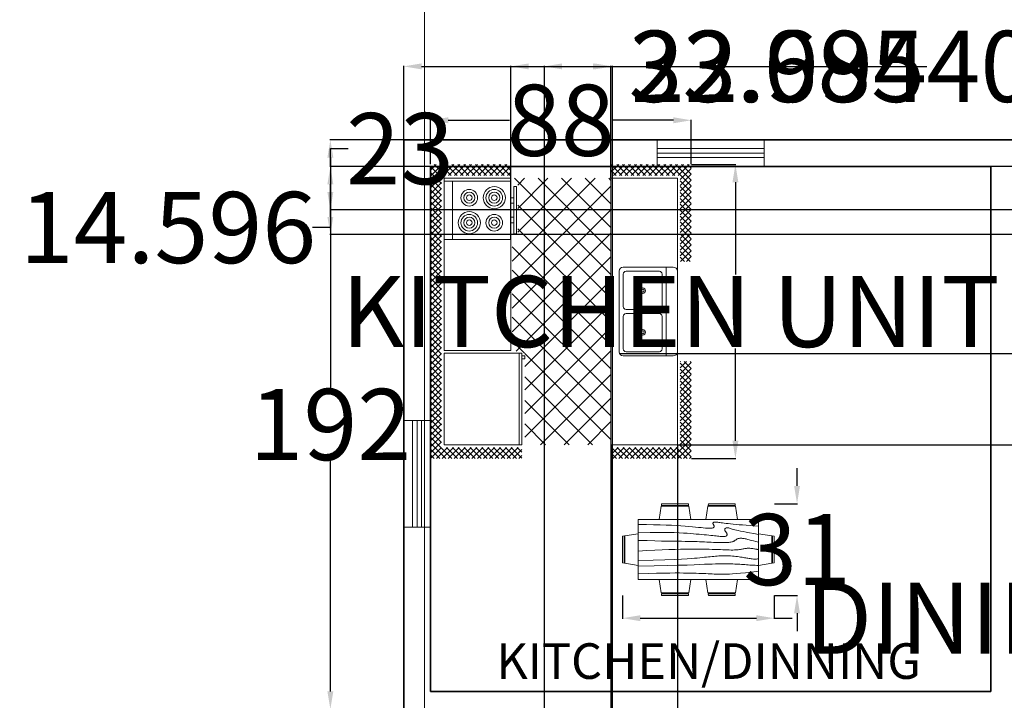
# Model space of a CAD drawing. Units: inches. Extents: x -15 to 1815, y 1023 to 2303.
# Tile 3 of 8: x 190 to 522, y 2069 to 2299. Entities that reach past the tile are written whole.
import ezdxf

# ---------------------------------------------------------------- set-up
doc = ezdxf.new("R2010")
doc.units = ezdxf.units.IN
doc.header["$MEASUREMENT"] = 0
for name, color, linetype, lineweight in [('A-ANNO-DIMS', 2, 'Continuous', 18), ('A-AREA-IDEN', 7, 'Continuous', 18), ('A-FLOR-FIXT', 9, 'Continuous', 18), ('A-FURN', 8, 'Continuous', 18), ('A-GLAZ', 4, 'Continuous', 18), ('A-REFR', 8, 'Continuous', 13), ('A-WALL', 7, 'Continuous', 35)]:
    doc.layers.add(name, color=color, linetype=linetype, lineweight=lineweight)
doc.styles.get("Standard").update_dxf_attribs({"font": 'arial.ttf'})
doc.dimstyles.get("Standard").update_dxf_attribs({"dimtxt": 24, "dimasz": 6, "dimexe": 0.18, "dimexo": 0.0625, "dimgap": 0.09, "dimtad": 0, "dimtih": 1, "dimtoh": 1, "dimdec": 0, "dimzin": 0, "dimdsep": 46, "dimlunit": 3, "dimtxsty": 'Standard', "dimcen": 0.09, "dimadec": 0, "dimazin": 0, "dimtfac": 1, "dimtdec": 0, "dimtofl": 0, "dimtmove": 0, "dimatfit": 3, "dimfxl": 1, "dimtolj": 1, "dimtzin": 0, "dimarcsym": 0})

# ---------------------------------------------------------------- blocks, each defined once
blk = doc.blocks.new('Dining Set - 36 x 72 in.')
for p, q in [((-22.2343, 26.00059), (-23.4847, 17.99762)), ((-22.2304, 26), (-5.7608, 26)), ((-22, 27.5), (-22.1562, 26.50042)), ((-5.8416, 26.5), (-22.1534, 26.5)), ((-22, 27.5), (-6, 27.5)), ((-5.8437, 26.49966), (-6, 27.5)), ((-4.5152, 17.99762), (-5.7655, 25.99926)), ((5.7657, 26.00059), (4.5153, 17.99762)), ((5.7696, 26), (22.2392, 26)), ((6, 27.5), (5.8438, 26.50042)), ((22.1584, 26.5), (5.8466, 26.5)), ((6, 27.5), (22, 27.5)), ((22.1563, 26.49966), (22, 27.5)), ((23.4848, 17.99762), (22.2345, 25.99926)), ((36, 18), (-36, 18)), ((-36, 18), (-36, -18)), ((36, -18), (36, 18)), ((-45.5, 8), (-44.5004, 8.15617)), ((-45.5, 8), (-45.5, -8)), ((-44.5, -8.15843), (-44.5, 8.15338)), ((-44.0006, 8.23428), (-35.9976, 9.48474)), ((-44, 8.23041), (-44, -8.23915)), ((44.0006, 8.23428), (35.9976, 9.48474)), ((44, 8.23041), (44, -8.23915)), ((44.5, -8.15843), (44.5, 8.15338)), ((45.5, 8), (44.5005, 8.15617)), ((45.5, 8), (45.5, -8)), ((-44.4997, -8.15631), (-45.5, -8)), ((-35.9976, -9.48476), (-43.9993, -8.2345)), ((35.9976, -9.48476), (43.9993, -8.2345)), ((44.4997, -8.15631), (45.5, -8)), ((-36, -18), (36, -18)), ((-22.2343, -26.0006), (-23.4847, -17.99762)), ((-4.5152, -17.99762), (-5.7655, -25.99928)), ((5.7657, -26.0006), (4.5153, -17.99762)), ((23.4848, -17.99762), (22.2345, -25.99928)), ((-22.2304, -26), (-5.7608, -26)), ((-22, -27.5), (-22.1562, -26.50044)), ((-5.8416, -26.5), (-22.1534, -26.5)), ((-22, -27.5), (-6, -27.5)), ((-5.8437, -26.49967), (-6, -27.5)), ((5.7696, -26), (22.2392, -26)), ((6, -27.5), (5.8438, -26.50044)), ((22.1584, -26.5), (5.8466, -26.5)), ((6, -27.5), (22, -27.5)), ((22.1563, -26.49967), (22, -27.5))]:
    blk.add_line(p, q)
for points in [[(-36, 15), (-31.1772, 14.97754), (-26.8079, 14.91406), (-22.8538, 14.81543), (-19.276, 14.6875), (-16.0362, 14.53613), (-13.0957, 14.36718), (-10.4159, 14.18652), (-7.9583, 14), (-5.6904, 13.81315), (-3.6035, 13.63021), (-1.6954, 13.45508), (0.0365, 13.29166), (1.5945, 13.14388), (2.9811, 13.01562), (4.1988, 12.9108), (5.25, 12.83333), (6.1393, 12.78613), (6.8802, 12.76823), (7.4883, 12.77767), (7.9792, 12.8125), (8.3685, 12.87077), (8.6719, 12.95052), (8.9049, 13.0498), (9.0833, 13.16666), (9.2205, 13.29899), (9.3216, 13.44401), (9.3895, 13.59879), (9.4271, 13.76041), (9.4373, 13.92594), (9.4232, 14.09245), (9.3875, 14.257), (9.3333, 14.41666), (9.2638, 14.56917), (9.1836, 14.71484), (9.0975, 14.85465), (9.0104, 14.98958), (8.9272, 15.1206), (8.8529, 15.2487), (8.7922, 15.37483), (8.75, 15.5), (8.7305, 15.62467), (8.7344, 15.74739), (8.7617, 15.86621), (8.8125, 15.97916), (8.8867, 16.08431), (8.9844, 16.17968), (9.1055, 16.26334), (9.25, 16.33333), (9.4189, 16.38802), (9.6172, 16.42708), (9.8506, 16.45052), (10.125, 16.45833), (10.4463, 16.45052), (10.8203, 16.42708), (11.2529, 16.38802), (11.75, 16.33333), (12.3184, 16.26318), (12.9694, 16.17838), (13.7151, 16.07991), (14.5677, 15.96875), (15.5395, 15.84586), (16.6426, 15.71224), (17.8893, 15.56884), (19.2917, 15.41666), (20.859, 15.25667), (22.5879, 15.08984), (24.4721, 14.91715), (26.5052, 14.73958), (28.6809, 14.5581), (30.9929, 14.3737), (33.4347, 14.18733), (36, 14)], [(-36, 10), (-28.9766, 10.14274), (-23.1725, 10.20442), (-18.4241, 10.19775), (-14.5677, 10.13541), (-11.4399, 10.03011), (-8.877, 9.89453), (-6.7154, 9.74137), (-4.7917, 9.58333), (-2.9698, 9.43082), (-1.2246, 9.28515), (0.4415, 9.14534), (2.026, 9.01041), (3.5266, 8.87939), (4.9408, 8.7513), (6.266, 8.62516), (7.5, 8.5), (8.6411, 8.37549), (9.6914, 8.2539), (10.6538, 8.13818), (11.5312, 8.03125), (12.3267, 7.93603), (13.043, 7.85547), (13.6831, 7.79248), (14.25, 7.75), (14.7471, 7.7303), (15.1797, 7.73307), (15.5537, 7.75732), (15.875, 7.80208), (16.1494, 7.86637), (16.3828, 7.94922), (16.5811, 8.04964), (16.75, 8.16666), (16.8944, 8.29915), (17.0143, 8.44531), (17.1089, 8.60319), (17.1771, 8.77083), (17.218, 8.94629), (17.2305, 9.1276), (17.2137, 9.31282), (17.1667, 9.5), (17.0895, 9.6875), (16.987, 9.875), (16.8649, 10.0625), (16.7292, 10.25), (16.5856, 10.4375), (16.4401, 10.625), (16.2985, 10.8125), (16.1667, 11), (16.05, 11.18733), (15.9518, 11.3737), (15.8752, 11.5581), (15.8229, 11.73958), (15.798, 11.91715), (15.8034, 12.08984), (15.842, 12.25667), (15.9167, 12.41666), (16.0295, 12.56836), (16.1784, 12.70833), (16.3605, 12.83268), (16.5729, 12.9375), (16.8127, 13.01888), (17.0768, 13.07291), (17.3625, 13.0957), (17.6667, 13.08333), (17.9894, 13.03312), (18.3418, 12.94726), (18.7382, 12.82918), (19.1927, 12.68229), (19.7195, 12.51001), (20.3327, 12.31575), (21.0465, 12.10294), (21.875, 11.875), (22.8357, 11.63354), (23.959, 11.37304), (25.2786, 11.08618), (26.8282, 10.76562), (28.6414, 10.40405), (30.752, 9.99414), (33.1936, 9.52856), (36, 9)], [(-36, 5.5), (-30.7157, 5.3348), (-26.069, 5.20963), (-21.9946, 5.11767), (-18.4271, 5.05208), (-15.3009, 5.00602), (-12.5508, 4.97265), (-10.1112, 4.94515), (-7.9167, 4.91666), (-5.909, 4.88167), (-4.0586, 4.83984), (-2.3429, 4.79215), (-0.7396, 4.73958), (0.7739, 4.6831), (2.22, 4.6237), (3.6213, 4.56233), (5, 4.5), (6.373, 4.43782), (7.7344, 4.3776), (9.0723, 4.32129), (10.375, 4.27083), (11.6309, 4.22819), (12.8281, 4.19531), (13.9551, 4.17415), (15, 4.16666), (15.954, 4.17448), (16.819, 4.19791), (17.6001, 4.23698), (18.3021, 4.29166), (18.9299, 4.36198), (19.4883, 4.44791), (19.9823, 4.54948), (20.4167, 4.66666), (20.7969, 4.79899), (21.1302, 4.94401), (21.4245, 5.09879), (21.6875, 5.26041), (21.9271, 5.42594), (22.1511, 5.59245), (22.3672, 5.757), (22.5834, 5.91666), (22.8065, 6.06868), (23.0404, 6.21093), (23.2879, 6.34147), (23.5521, 6.45833), (23.8358, 6.55957), (24.142, 6.64323), (24.4735, 6.70735), (24.8334, 6.75), (25.2235, 6.76969), (25.642, 6.76692), (26.0858, 6.74267), (26.5521, 6.69791), (27.0379, 6.63362), (27.5404, 6.55078), (28.0565, 6.45036), (28.5834, 6.33333), (29.1242, 6.19987), (29.7071, 6.04687), (30.3661, 5.87044), (31.1354, 5.66666), (32.0493, 5.43164), (33.142, 5.16146), (34.4475, 4.85221), (36, 4.5)], [(-36, -1), (-30.7915, -0.6591), (-26.0195, -0.38216), (-21.6519, -0.16284), (-17.6563, 0.00521), (-14.0005, 0.12833), (-10.6523, 0.21289), (-7.5796, 0.26522), (-4.75, 0.29166), (-2.134, 0.29793), (0.2878, 0.28711), (2.5317, 0.26163), (4.6146, 0.22396), (6.5529, 0.17651), (8.3633, 0.12174), (10.0623, 0.06209), (11.6667, 0), (13.1899, -0.06201), (14.6341, -0.1211), (15.9982, -0.17432), (17.2813, -0.21875), (18.4823, -0.25147), (19.6003, -0.26953), (20.6343, -0.27002), (21.5834, -0.25), (22.4481, -0.20768), (23.2357, -0.14584), (23.9549, -0.06836), (24.6146, 0.02083), (25.2235, 0.11784), (25.7904, 0.21875), (26.3241, 0.31966), (26.8334, 0.41666), (27.3265, 0.50618), (27.8099, 0.58593), (28.2894, 0.65397), (28.7709, 0.70833), (29.2601, 0.74707), (29.763, 0.76823), (30.2855, 0.76985), (30.8334, 0.75), (31.4088, 0.70784), (31.9994, 0.64713), (32.589, 0.57275), (33.1615, 0.48958), (33.7008, 0.4025), (34.1908, 0.3164), (34.6153, 0.23616), (34.9584, 0.16666), (35.2099, 0.11165), (35.3848, 0.07031), (35.504, 0.04069), (35.5886, 0.02083), (35.6594, 0.00879), (35.7377, 0.0026), (35.8442, 0.00032), (36, 0)], [(-36, -6.5), (-27.1843, -6.31267), (-20.084, -6.1263), (-14.469, -5.9419), (-10.1094, -5.76042), (-6.7752, -5.58285), (-4.2363, -5.41016), (-2.2629, -5.24333), (-0.625, -5.08334), (0.8708, -4.93099), (2.2715, -4.78646), (3.5872, -4.64974), (4.8281, -4.52084), (6.0046, -4.39974), (7.127, -4.28646), (8.2053, -4.18099), (9.25, -4.08334), (10.2705, -3.99382), (11.2734, -3.91407), (12.2647, -3.84603), (13.25, -3.79167), (14.2354, -3.75293), (15.2266, -3.73177), (16.2295, -3.73015), (17.25, -3.75), (18.2912, -3.79248), (19.3451, -3.85547), (20.4009, -3.93604), (21.4479, -4.03125), (22.4754, -4.13819), (23.4727, -4.25391), (24.4289, -4.37549), (25.3334, -4.5), (26.1785, -4.62492), (26.9694, -4.74935), (27.7145, -4.87281), (28.4219, -4.99479), (29.1, -5.11483), (29.7572, -5.23242), (30.4016, -5.34709), (31.0417, -5.45834), (31.6837, -5.56437), (32.3262, -5.65821), (32.9658, -5.73153), (33.599, -5.77604), (34.2224, -5.78345), (34.8327, -5.74545), (35.4264, -5.65373), (36, -5.5)], [(-36, -10), (-26.4022, -9.81299), (-18.4675, -9.62891), (-11.9839, -9.45069), (-6.7396, -9.28125), (-2.5226, -9.12354), (0.8789, -8.98047), (3.6769, -8.85498), (6.0833, -8.75), (8.2767, -8.66765), (10.3021, -8.60677), (12.1712, -8.56543), (13.8958, -8.54167), (15.4876, -8.53353), (16.9583, -8.53907), (18.3197, -8.55632), (19.5834, -8.58334), (20.7616, -8.61841), (21.8685, -8.66081), (22.9188, -8.71004), (23.9271, -8.76563), (24.9081, -8.82707), (25.8763, -8.89388), (26.8465, -8.96558), (27.8334, -9.04167), (28.8474, -9.12118), (29.8828, -9.20117), (30.93, -9.27824), (31.9792, -9.34896), (33.0205, -9.40991), (34.0443, -9.45768), (35.0407, -9.48885), (36, -9.5)], [(-36, -14.5), (-30.0881, -14.33513), (-25.0332, -14.21224), (-20.7312, -14.12647), (-17.0781, -14.07292), (-13.97, -14.04671), (-11.3027, -14.04297), (-8.9724, -14.05681), (-6.875, -14.08334), (-4.9224, -14.11833), (-3.0905, -14.16016), (-1.3709, -14.20785), (0.2448, -14.26042), (1.7647, -14.3169), (3.1973, -14.3763), (4.5507, -14.43767), (5.8333, -14.5), (7.0554, -14.5621), (8.235, -14.62175), (9.3922, -14.67652), (10.5469, -14.72396), (11.7192, -14.76164), (12.929, -14.78711), (14.1965, -14.79794), (15.5417, -14.79167), (16.9933, -14.76424), (18.6152, -14.70508), (20.4804, -14.60197), (22.6615, -14.44271), (25.2312, -14.21509), (28.2624, -13.9069), (31.8277, -13.50594), (36, -13)]]:
    blk.add_lwpolyline(points)
blk = doc.blocks.new('Kitchen Layout - 7 x 8 ft')
for p, q in [((-5, 81.32), (2.68, 89)), ((-5, 83.44), (0.56, 89)), ((-5, 85.56), (-1.56, 89)), ((-5, 87.68), (-3.68, 89)), ((-1, 84.97), (-5, 88.97)), ((1.09, 85), (-2.91, 89)), ((3.21, 85), (-0.79, 89)), ((0.81, 85), (4.81, 89)), ((5.34, 85), (1.34, 89)), ((2.93, 85), (6.93, 89)), ((7.46, 85), (3.46, 89)), ((5.05, 85), (9.05, 89)), ((9.58, 85), (5.58, 89)), ((7.17, 85), (11.17, 89)), ((11.7, 85), (7.7, 89)), ((9.29, 85), (13.29, 89)), ((13.82, 85), (9.82, 89)), ((11.41, 85), (15.41, 89)), ((15.94, 85), (11.94, 89)), ((13.53, 85), (17.53, 89)), ((18.06, 85), (14.06, 89)), ((15.65, 85), (19.65, 89)), ((20.18, 85), (16.18, 89)), ((17.78, 85), (21.78, 89)), ((22.31, 85), (18.31, 89)), ((19.9, 85), (23.9, 89)), ((24.43, 85), (20.43, 89)), ((22.02, 85), (26.02, 89)), ((26.55, 85), (22.55, 89)), ((24.14, 85), (28.14, 89)), ((28.67, 85), (24.67, 89)), ((26.26, 85), (30.26, 89)), ((30.79, 85), (26.79, 89)), ((28.38, 85), (32.38, 89)), ((32.91, 85), (28.91, 89)), ((30.5, 85), (34.5, 89)), ((35.03, 85), (31.03, 89)), ((32.63, 85), (36.63, 89)), ((37.16, 85), (33.16, 89)), ((34.75, 85), (38.75, 89)), ((39.28, 85), (35.28, 89)), ((36.87, 85), (40.87, 89)), ((41.4, 85), (37.4, 89)), ((38.99, 85), (42.99, 89)), ((43.52, 85), (39.52, 89)), ((41.11, 85), (45.11, 89)), ((45.64, 85), (41.64, 89)), ((43.23, 85), (47.23, 89)), ((47.76, 85), (43.76, 89)), ((45.35, 85), (49.35, 89)), ((49.88, 85), (45.88, 89)), ((47.47, 85), (51.47, 89)), ((52, 85), (48, 89)), ((49.6, 85), (53.6, 89)), ((54.13, 85), (50.13, 89)), ((51.72, 85), (55.72, 89)), ((56.25, 85), (52.25, 89)), ((53.84, 85), (57.84, 89)), ((58.37, 85), (54.37, 89)), ((55.96, 85), (59.96, 89)), ((60.49, 85), (56.49, 89)), ((58.08, 85), (62.08, 89)), ((62.61, 85), (58.61, 89)), ((60.2, 85), (64.2, 89)), ((64.73, 85), (60.73, 89)), ((62.32, 85), (66.32, 89)), ((66.85, 85), (62.85, 89)), ((64.45, 85), (68.45, 89)), ((68.97, 85), (64.97, 89)), ((66.57, 85), (70.57, 89)), ((71.1, 85), (67.1, 89)), ((68.69, 85), (72.69, 89)), ((73.22, 85), (69.22, 89)), ((70.81, 85), (74.81, 89)), ((75.34, 85), (71.34, 89)), ((72.93, 85), (76.93, 89)), ((77.46, 85), (73.46, 89)), ((75.05, 85), (79.05, 89)), ((79.58, 85), (75.58, 89)), ((77.17, 85), (81.17, 89)), ((81.7, 85), (77.7, 89)), ((79.29, 85), (83.29, 89)), ((83.82, 85), (79.82, 89)), ((81.42, 85), (85.42, 89)), ((85.95, 85), (81.95, 89)), ((83.54, 85), (87.54, 89)), ((88.07, 85), (84.07, 89)), ((85.66, 85), (89.66, 89)), ((90.19, 85), (86.19, 89)), ((87.78, 85), (91.78, 89)), ((92.31, 85), (88.31, 89)), ((89.9, 85), (93.9, 89)), ((94.43, 85), (90.43, 89)), ((92.02, 85), (96.02, 89)), ((96.55, 85), (92.55, 89)), ((94.14, 85), (98.14, 89)), ((101, 82.67), (94.67, 89)), ((96.27, 85), (100.27, 89)), ((101, 84.79), (96.79, 89)), ((101, 86.92), (98.92, 89)), ((-1, 82.85), (-5, 86.85)), ((97, 83.61), (101, 87.61)), ((97, 81.49), (101, 85.49)), ((-1, 80.73), (-5, 84.73)), ((-5, 79.19), (-1, 83.19)), ((-1, 78.61), (-5, 82.61)), ((34, 84), (96, 84)), ((34, 60), (34, 84)), ((96, 84), (96, 60)), ((101, 80.55), (97, 84.55)), ((97, 79.37), (101, 83.37)), ((101, 78.43), (97, 82.43)), ((-5, 77.07), (-1, 81.07)), ((-1, 76.49), (-5, 80.49)), ((-5, 74.95), (-1, 78.95)), ((-1, 74.36), (-5, 78.36)), ((74, 81), (95, 81)), ((97, 77.25), (101, 81.25)), ((101, 76.31), (97, 80.31)), ((97, 75.13), (101, 79.13)), ((101, 74.19), (97, 78.19)), ((-5, 72.83), (-1, 76.83)), ((-1, 72.24), (-5, 76.24)), ((-5, 70.71), (-1, 74.71)), ((97, 73.01), (101, 77.01)), ((101, 72.07), (97, 76.07)), ((97, 70.89), (101, 74.89)), ((-1, 70.12), (-5, 74.12)), ((-5, 68.59), (-1, 72.59)), ((-1, 68), (-5, 72)), ((101, 69.95), (97, 73.95)), ((97, 68.76), (101, 72.76)), ((101, 67.82), (97, 71.82)), ((-5, 66.47), (-1, 70.47)), ((-1, 65.88), (-5, 69.88)), ((-5, 64.35), (-1, 68.35)), ((-1, 63.76), (-5, 67.76)), ((97, 66.64), (101, 70.64)), ((101, 65.7), (97, 69.7)), ((97, 64.52), (101, 68.52)), ((101, 63.58), (97, 67.58)), ((-5, 62.22), (-1, 66.22)), ((-1, 61.64), (-5, 65.64)), ((-5, 60.1), (-1, 64.1)), ((97, 62.4), (101, 66.4)), ((101, 61.46), (97, 65.46)), ((97, 60.28), (101, 64.28)), ((-1, 59.52), (-5, 63.52)), ((-5, 57.98), (-1, 61.98)), ((-1, 57.39), (-5, 61.39)), ((100.34, 60), (97, 63.34)), ((98.22, 60), (97, 61.22)), ((98.84, 60), (101, 62.16)), ((-1.73, 56), (-5, 59.27)), ((-3.85, 56), (-5, 57.15)), ((-4.86, 56), (-1, 59.86)), ((-2.74, 56), (-1, 57.74)), ((0, 57), (33, 57)), ((10.4, 24), (45.9, 59.5)), ((18.88, 24), (54.38, 59.5)), ((27.37, 24), (62.87, 59.5)), ((33.03, 55.11), (37.41, 59.5)), ((67.71, 24), (33.68, 58.04)), ((96, 60), (34, 60)), ((35.85, 24), (71.35, 59.5)), ((76.2, 24), (40.7, 59.5)), ((44.34, 24), (77.84, 57.5)), ((84.68, 24), (49.18, 59.5)), ((52.82, 24), (86.32, 57.5)), ((93.17, 24), (57.67, 59.5)), ((61.31, 24), (96, 58.69)), ((96, 29.65), (66.15, 59.5)), ((96, 38.14), (76.64, 57.5)), ((80, 60), (80, 59)), ((82, 59), (82, 60)), ((96, 46.63), (85.13, 57.5)), ((87, 59), (87, 60)), ((89, 60), (89, 59)), ((96, 55.11), (93.57, 57.54)), ((100.96, 60), (101, 60.04)), ((0, 30.57), (24.43, 55)), ((0, 39.06), (15.94, 55)), ((0, 47.54), (7.46, 55)), ((1.91, 24), (32.91, 55)), ((33.77, 24), (2.77, 55)), ((42.26, 24), (11.26, 55)), ((50.74, 24), (19.74, 55)), ((59.23, 24), (28.23, 55)), ((31, 55), (31, 56)), ((32, 55), (31, 55)), ((32, 56), (32, 55)), ((69.79, 24), (96, 50.21)), ((25.29, 24), (0, 49.29)), ((16.8, 24), (0, 40.8)), ((78.28, 24), (96, 41.72)), ((8.32, 24), (0, 32.32)), ((86.76, 24), (96, 33.24)), ((-5, 21.92), (-2.92, 24)), ((-5, 19.8), (-1, 23.8)), ((-1, 19.21), (-5, 23.21)), ((-5, 17.68), (-1, 21.68)), ((-1, 21.33), (-3.67, 24)), ((-1, 23.45), (-1.55, 24)), ((0, 24), (96, 24)), ((0, 0), (0, 24)), ((95.25, 24), (96, 24.75)), ((96, 24), (96, 0)), ((97, 22.1), (98.9, 24)), ((97, 19.97), (101, 23.97)), ((101, 19.03), (97, 23.03)), ((97, 17.85), (101, 21.85)), ((101, 21.16), (98.16, 24)), ((101, 23.28), (100.28, 24)), ((-1, 17.09), (-5, 21.09)), ((-5, 15.55), (-1, 19.55)), ((-1, 14.97), (-5, 18.97)), ((47.25, 6.5), (47.25, 18.5)), ((48.75, 18.5), (48.75, 6.5)), ((101, 16.91), (97, 20.91)), ((97, 15.73), (101, 19.73)), ((101, 14.79), (97, 18.79)), ((-5, 13.43), (-1, 17.43)), ((-1, 12.85), (-5, 16.85)), ((-5, 11.31), (-1, 15.31)), ((-1, 10.73), (-5, 14.73)), ((97, 13.61), (101, 17.61)), ((101, 12.67), (97, 16.67)), ((97, 11.49), (101, 15.49)), ((101, 10.55), (97, 14.55)), ((-5, 9.19), (-1, 13.19)), ((-1, 8.6), (-5, 12.6)), ((-5, 7.07), (-1, 11.07)), ((97, 9.37), (101, 13.37)), ((101, 8.43), (97, 12.43)), ((97, 7.25), (101, 11.25)), ((-1, 6.48), (-5, 10.48)), ((-5, 4.95), (-1, 8.95)), ((-1, 4.36), (-5, 8.36)), ((101, 6.31), (97, 10.31)), ((97, 5.12), (101, 9.12)), ((101, 4.18), (97, 8.18)), ((-5, 2.83), (-1, 6.83)), ((-1, 2.24), (-5, 6.24)), ((-5, 0.71), (-1, 4.71)), ((-1, 0.12), (-5, 4.12)), ((64, 4), (32, 4)), ((97, 3), (101, 7)), ((101, 2.06), (97, 6.06)), ((97, 0.88), (101, 4.88)), ((101, -0.06), (97, 3.94)), ((-5, -1.42), (-1, 2.58)), ((2, -5), (-5, 2)), ((-5, -3.54), (-1, 0.46)), ((96, 0), (0, 0)), ((93.24, -5), (101, 2.76)), ((95.36, -5), (101, 0.64)), ((101, -2.18), (97, 1.82)), ((-0.12, -5), (-5, -0.12)), ((-2.25, -5), (-5, -2.25)), ((-4.34, -5), (-0.34, -1)), ((-2.22, -5), (1.78, -1)), ((-0.1, -5), (3.9, -1)), ((4.12, -5), (0.12, -1)), ((2.02, -5), (6.02, -1)), ((6.24, -5), (2.24, -1)), ((4.14, -5), (8.14, -1)), ((8.36, -5), (4.36, -1)), ((6.27, -5), (10.27, -1)), ((10.48, -5), (6.48, -1)), ((8.39, -5), (12.39, -1)), ((12.6, -5), (8.6, -1)), ((10.51, -5), (14.51, -1)), ((14.73, -5), (10.73, -1)), ((12.63, -5), (16.63, -1)), ((16.85, -5), (12.85, -1)), ((14.75, -5), (18.75, -1)), ((18.97, -5), (14.97, -1)), ((16.87, -5), (20.87, -1)), ((21.09, -5), (17.09, -1)), ((18.99, -5), (22.99, -1)), ((23.21, -5), (19.21, -1)), ((21.11, -5), (25.11, -1)), ((25.33, -5), (21.33, -1)), ((23.24, -5), (27.24, -1)), ((27.45, -5), (23.45, -1)), ((25.36, -5), (29.36, -1)), ((29.57, -5), (25.57, -1)), ((27.48, -5), (30, -2.48)), ((30, -3.3), (27.7, -1)), ((30, -1.18), (29.82, -1)), ((66, -2.54), (67.54, -1)), ((66, -4.66), (69.66, -1)), ((69.88, -5), (66, -1.12)), ((67.76, -5), (66, -3.24)), ((67.78, -5), (71.78, -1)), ((72, -5), (68, -1)), ((69.9, -5), (73.9, -1)), ((74.12, -5), (70.12, -1)), ((72.03, -5), (76.03, -1)), ((76.24, -5), (72.24, -1)), ((74.15, -5), (78.15, -1)), ((78.36, -5), (74.36, -1)), ((76.27, -5), (80.27, -1)), ((80.49, -5), (76.49, -1)), ((78.39, -5), (82.39, -1)), ((82.61, -5), (78.61, -1)), ((80.51, -5), (84.51, -1)), ((84.73, -5), (80.73, -1)), ((82.63, -5), (86.63, -1)), ((86.85, -5), (82.85, -1)), ((84.75, -5), (88.75, -1)), ((88.97, -5), (84.97, -1)), ((86.88, -5), (90.88, -1)), ((91.09, -5), (87.09, -1)), ((89, -5), (93, -1)), ((93.21, -5), (89.21, -1)), ((91.12, -5), (95.12, -1)), ((95.34, -5), (91.34, -1)), ((97.46, -5), (93.46, -1)), ((99.58, -5), (95.58, -1)), ((101, -4.3), (97, -0.3)), ((97.48, -5), (101, -1.48)), ((-4.37, -5), (-5, -4.37)), ((29.6, -5), (30, -4.6)), ((99.6, -5), (101, -3.6))]:
    blk.add_line(p, q)
for points in [[(0, 56), (0, 84), (33, 84), (33, 56)], [(74, 60), (74, 84), (95, 84), (95, 60)], [(76, 58), (76, 59), (93, 59), (93, 58)]]:
    blk.add_lwpolyline(points, close=True)
for points in [[(32, 1.5), (32, 19.5)], [(33.5, 21), (62.5, 21)], [(33.5, 6.5), (33.5, 18.5)], [(34.5, 19.5), (46.25, 19.5)], [(49.75, 19.5), (61.5, 19.5)], [(62.5, 18.5), (62.5, 6.5)], [(64, 19.5), (64, 1.5)], [(46.25, 5.5), (34.5, 5.5)], [(61.5, 5.5), (49.75, 5.5)], [(62.5, 0), (33.5, 0)]]:
    blk.add_lwpolyline(points)
for centre, radius in [((80, 75), 4), ((80, 75), 3), ((80, 75), 2), ((80, 75), 1), ((89, 75), 3), ((89, 75), 2), ((89, 75), 1), ((80, 66), 3), ((80, 66), 2), ((89, 66), 4), ((89, 66), 3), ((89, 66), 2), ((80, 66), 1), ((89, 66), 1), ((40.5, 12.5), 1), ((40.5, 12.5), 0.5), ((55.5, 12.5), 1), ((55.5, 12.5), 0.5)]:
    blk.add_circle(centre, radius)
for centre, radius, start, end in [((33.5, 19.5), 1.5, 90, 180), ((34.5, 18.5), 1, 90, 180), ((46.25, 18.5), 1, 0, 90), ((49.75, 18.5), 1, 90, 180), ((61.5, 18.5), 1, 0, 90), ((62.5, 19.5), 1.5, 0, 90), ((34.5, 6.5), 1, 180, 270), ((46.25, 6.5), 1, 270, 0), ((49.75, 6.5), 1, 180, 270), ((61.5, 6.5), 1, 270, 0), ((33.5, 1.5), 1.5, 180, 270), ((62.5, 1.5), 1.5, 270, 0)]:
    blk.add_arc(centre, radius, start, end)
blk = doc.blocks.new('Window - Wood Frame 36 in. Wide plan')
for p, q in [((0, 7.5), (0, -1.5)), ((36, 7.5), (36, -1.5)), ((0, 4.5), (36, 4.5)), ((0, 3), (36, 3)), ((0, 1.5), (36, 1.5))]:
    blk.add_line(p, q)
blk = doc.blocks.new('*D33')
at = {"layer": 'A-ANNO-DIMS', "color": 0, "lineweight": -2, "transparency": 16777216}
for p, q in [((393.59, 2104.63), (393.59, 2096.83)), ((444.77, 2104.63), (444.77, 2096.83)), ((399.59, 2097.01), (438.77, 2097.01)), ((444.77, 2097.01), (450.77, 2097.01))]:
    blk.add_line(p, q, dxfattribs=at)
at = {"layer": 'A-ANNO-DIMS', "color": 0, "transparency": 16777216}
for points in [[(399.59, 2098.01), (399.59, 2096.01), (393.59, 2097.01)], [(438.77, 2098.01), (438.77, 2096.01), (444.77, 2097.01)]]:
    blk.add_solid(points, dxfattribs=at)
at = {"layer": 'Defpoints', "color": 0, "transparency": 16777216}
for p in [(393.59, 2104.69), (444.77, 2104.69), (444.77, 2097.01)]:
    blk.add_point(p, dxfattribs=at)
at = {"layer": 'A-ANNO-DIMS', "color": 0, "transparency": 16777216, "insert": (565.73, 2097.01), "char_height": 24, "attachment_point": 5}
blk.add_mtext('\\A1;DINING SET 51', dxfattribs=at)
blk = doc.blocks.new('*D34')
at = {"layer": 'A-ANNO-DIMS', "color": 0, "lineweight": -2, "transparency": 16777216}
for p, q in [((452.45, 2141.62), (452.45, 2147.62)), ((444.83, 2135.62), (452.63, 2135.62)), ((444.83, 2104.69), (452.63, 2104.69)), ((452.45, 2098.69), (452.45, 2092.69))]:
    blk.add_line(p, q, dxfattribs=at)
at = {"layer": 'A-ANNO-DIMS', "color": 0, "transparency": 16777216}
for points in [[(451.45, 2141.62), (453.45, 2141.62), (452.45, 2135.62)], [(451.45, 2098.69), (453.45, 2098.69), (452.45, 2104.69)]]:
    blk.add_solid(points, dxfattribs=at)
at = {"layer": 'Defpoints', "color": 0, "transparency": 16777216}
for p in [(444.77, 2135.62), (452.45, 2135.62), (444.77, 2104.69)]:
    blk.add_point(p, dxfattribs=at)
at = {"layer": 'A-ANNO-DIMS', "color": 0, "transparency": 16777216, "insert": (452.45, 2120.16), "char_height": 24, "attachment_point": 5}
blk.add_mtext('\\A1;31', dxfattribs=at)
blk = doc.blocks.new('*D39')
at = {"layer": 'A-ANNO-DIMS', "color": 0, "lineweight": -2, "transparency": 16777216}
for p, q in [((416.85, 2250.01), (431.85, 2250.01)), ((431.67, 2244.01), (431.67, 2212.92)), ((431.67, 2156.83), (431.67, 2187.92)), ((416.85, 2150.83), (431.85, 2150.83))]:
    blk.add_line(p, q, dxfattribs=at)
at = {"layer": 'A-ANNO-DIMS', "color": 0, "transparency": 16777216}
for points in [[(430.67, 2244.01), (432.67, 2244.01), (431.67, 2250.01)], [(430.67, 2156.83), (432.67, 2156.83), (431.67, 2150.83)]]:
    blk.add_solid(points, dxfattribs=at)
at = {"layer": 'Defpoints', "color": 0, "transparency": 16777216}
for p in [(416.79, 2250.01), (431.67, 2250.01), (416.79, 2150.83)]:
    blk.add_point(p, dxfattribs=at)
at = {"layer": 'A-ANNO-DIMS', "color": 0, "transparency": 16777216, "insert": (431.67, 2200.42), "char_height": 24, "attachment_point": 5}
blk.add_mtext('\\A1;KITCHEN UNIT 99', dxfattribs=at)
blk = doc.blocks.new('*D40')
at = {"layer": 'A-ANNO-DIMS', "color": 0, "lineweight": -2, "transparency": 16777216}
for p, q in [((328.83, 2250.08), (328.83, 2265.07)), ((334.83, 2264.89), (355.49, 2264.89)), ((410.79, 2264.89), (390.13, 2264.89)), ((416.79, 2250.08), (416.79, 2265.07))]:
    blk.add_line(p, q, dxfattribs=at)
at = {"layer": 'A-ANNO-DIMS', "color": 0, "transparency": 16777216}
for points in [[(334.83, 2265.89), (334.83, 2263.89), (328.83, 2264.89)], [(410.79, 2265.89), (410.79, 2263.89), (416.79, 2264.89)]]:
    blk.add_solid(points, dxfattribs=at)
at = {"layer": 'Defpoints', "color": 0, "transparency": 16777216}
for p in [(328.83, 2264.89), (328.83, 2250.01), (416.79, 2250.01)]:
    blk.add_point(p, dxfattribs=at)
at = {"layer": 'A-ANNO-DIMS', "color": 0, "transparency": 16777216, "insert": (372.81, 2264.89), "char_height": 24, "attachment_point": 5}
blk.add_mtext('\\A1;88', dxfattribs=at)
blk = doc.blocks.new('*D59')
at = {"layer": 'A-ANNO-DIMS', "color": 0, "lineweight": -2, "transparency": 16777216}
for p, q in [((319.83, 2258.39), (319.83, 2283.24)), ((325.83, 2283.06), (496.25, 2283.06)), ((720.83, 2283.06), (550.42, 2283.06)), ((726.83, 2258.39), (726.83, 2283.24))]:
    blk.add_line(p, q, dxfattribs=at)
at = {"layer": 'A-ANNO-DIMS', "color": 0, "transparency": 16777216}
for points in [[(325.83, 2284.06), (325.83, 2282.06), (319.83, 2283.06)], [(720.83, 2284.06), (720.83, 2282.06), (726.83, 2283.06)]]:
    blk.add_solid(points, dxfattribs=at)
at = {"layer": 'Defpoints', "color": 0, "transparency": 16777216}
for p in [(726.83, 2283.06), (319.83, 2258.33), (726.83, 2258.33)]:
    blk.add_point(p, dxfattribs=at)
at = {"layer": 'A-ANNO-DIMS', "color": 0, "transparency": 16777216, "insert": (523.33, 2283.06), "char_height": 24, "attachment_point": 5}
blk.add_mtext('\\A1;407', dxfattribs=at)
blk = doc.blocks.new('*D63')
at = {"layer": 'A-ANNO-DIMS', "color": 0, "lineweight": -2, "transparency": 16777216}
for p, q in [((319.77, 2258.33), (294.92, 2258.33)), ((295.1, 2252.33), (295.1, 2174.67)), ((295.1, 2072.33), (295.1, 2149.98)), ((319.77, 2066.33), (294.92, 2066.33))]:
    blk.add_line(p, q, dxfattribs=at)
at = {"layer": 'A-ANNO-DIMS', "color": 0, "transparency": 16777216}
for points in [[(294.1, 2252.33), (296.1, 2252.33), (295.1, 2258.33)], [(294.1, 2072.33), (296.1, 2072.33), (295.1, 2066.33)]]:
    blk.add_solid(points, dxfattribs=at)
at = {"layer": 'Defpoints', "color": 0, "transparency": 16777216}
for p in [(295.1, 2258.33), (319.83, 2258.33), (319.83, 2066.33)]:
    blk.add_point(p, dxfattribs=at)
at = {"layer": 'A-ANNO-DIMS', "color": 0, "transparency": 16777216, "insert": (295.1, 2162.33), "char_height": 24, "attachment_point": 5}
blk.add_mtext('\\A1;192', dxfattribs=at)
blk = doc.blocks.new('*D68')
at = {"layer": 'A-ANNO-DIMS', "color": 0, "lineweight": -2, "transparency": 16777216}
for p, q in [((367.25, 1964.98), (367.25, 2283.24)), ((373.25, 2283.06), (384.24, 2283.06)), ((390.24, 1945.2), (390.24, 2283.24)), ((390.24, 2283.06), (396.24, 2283.06))]:
    blk.add_line(p, q, dxfattribs=at)
at = {"layer": 'A-ANNO-DIMS', "color": 0, "transparency": 16777216}
for points in [[(373.25, 2284.06), (373.25, 2282.06), (367.25, 2283.06)], [(384.24, 2284.06), (384.24, 2282.06), (390.24, 2283.06)]]:
    blk.add_solid(points, dxfattribs=at)
at = {"layer": 'Defpoints', "color": 0, "transparency": 16777216}
for p in [(390.24, 2283.06), (367.25, 1964.92), (390.24, 1945.14)]:
    blk.add_point(p, dxfattribs=at)
at = {"layer": 'A-ANNO-DIMS', "color": 0, "transparency": 16777216, "insert": (446.3, 2283.06), "char_height": 24, "attachment_point": 5}
blk.add_mtext('\\A1;22.994', dxfattribs=at)
blk = doc.blocks.new('*D74')
at = {"layer": 'A-ANNO-DIMS', "color": 0, "lineweight": -2, "transparency": 16777216}
for p, q in [((295.1, 2249.33), (295.1, 2255.33)), ((295.1, 2255.33), (301.1, 2255.33)), ((623.77, 2249.33), (294.92, 2249.33)), ((295.1, 2232.33), (295.1, 2243.33)), ((681.77, 2226.33), (294.92, 2226.33))]:
    blk.add_line(p, q, dxfattribs=at)
at = {"layer": 'A-ANNO-DIMS', "color": 0, "transparency": 16777216}
for points in [[(294.1, 2243.33), (296.1, 2243.33), (295.1, 2249.33)], [(294.1, 2232.33), (296.1, 2232.33), (295.1, 2226.33)]]:
    blk.add_solid(points, dxfattribs=at)
at = {"layer": 'Defpoints', "color": 0, "transparency": 16777216}
for p in [(295.1, 2249.33), (623.83, 2249.33), (681.83, 2226.33)]:
    blk.add_point(p, dxfattribs=at)
at = {"layer": 'A-ANNO-DIMS', "color": 0, "transparency": 16777216, "insert": (318.59, 2255.33), "char_height": 24, "attachment_point": 5}
blk.add_mtext('\\A1;23', dxfattribs=at)
blk = doc.blocks.new('*D76')
at = {"layer": 'A-ANNO-DIMS', "color": 0, "lineweight": -2, "transparency": 16777216}
for p, q in [((523.77, 2249.33), (294.92, 2249.33)), ((295.1, 2243.33), (295.1, 2240.73)), ((543.56, 2234.73), (294.92, 2234.73)), ((295.1, 2234.73), (295.1, 2228.73)), ((295.1, 2228.73), (289.1, 2228.73))]:
    blk.add_line(p, q, dxfattribs=at)
at = {"layer": 'A-ANNO-DIMS', "color": 0, "transparency": 16777216}
for points in [[(294.1, 2243.33), (296.1, 2243.33), (295.1, 2249.33)], [(294.1, 2240.73), (296.1, 2240.73), (295.1, 2234.73)]]:
    blk.add_solid(points, dxfattribs=at)
at = {"layer": 'Defpoints', "color": 0, "transparency": 16777216}
for p in [(523.83, 2249.33), (295.1, 2234.73), (543.62, 2234.73)]:
    blk.add_point(p, dxfattribs=at)
at = {"layer": 'A-ANNO-DIMS', "color": 0, "transparency": 16777216, "insert": (240.33, 2228.73), "char_height": 24, "attachment_point": 5}
blk.add_mtext('\\A1;14.596', dxfattribs=at)
blk = doc.blocks.new('*D77')
at = {"layer": 'A-ANNO-DIMS', "color": 0, "lineweight": -2, "transparency": 16777216}
for p, q in [((355.97, 2224.81), (355.97, 2283.24)), ((361.97, 2283.06), (383.65, 2283.06)), ((389.65, 2245.4), (389.65, 2283.24)), ((389.65, 2283.06), (395.65, 2283.06))]:
    blk.add_line(p, q, dxfattribs=at)
at = {"layer": 'A-ANNO-DIMS', "color": 0, "transparency": 16777216}
for points in [[(361.97, 2284.06), (361.97, 2282.06), (355.97, 2283.06)], [(383.65, 2284.06), (383.65, 2282.06), (389.65, 2283.06)]]:
    blk.add_solid(points, dxfattribs=at)
at = {"layer": 'Defpoints', "color": 0, "transparency": 16777216}
for p in [(389.65, 2283.06), (389.65, 2245.34), (355.97, 2224.75)]:
    blk.add_point(p, dxfattribs=at)
at = {"layer": 'A-ANNO-DIMS', "color": 0, "transparency": 16777216, "insert": (445.64, 2283.06), "char_height": 24, "attachment_point": 5}
blk.add_mtext('\\A1;33.685', dxfattribs=at)
blk = doc.blocks.new('*D78')
at = {"layer": 'A-ANNO-DIMS', "color": 0, "lineweight": -2, "transparency": 16777216}
for p, q in [((389.65, 2155.45), (389.65, 1800.41)), ((412.11, 2155.45), (412.11, 1800.41)), ((395.65, 1800.59), (406.11, 1800.59)), ((412.11, 1800.59), (418.11, 1800.59))]:
    blk.add_line(p, q, dxfattribs=at)
at = {"layer": 'A-ANNO-DIMS', "color": 0, "transparency": 16777216}
for points in [[(395.65, 1801.59), (395.65, 1799.59), (389.65, 1800.59)], [(406.11, 1801.59), (406.11, 1799.59), (412.11, 1800.59)]]:
    blk.add_solid(points, dxfattribs=at)
at = {"layer": 'Defpoints', "color": 0, "transparency": 16777216}
for p in [(389.65, 2155.51), (412.11, 2155.51), (412.11, 1800.59)]:
    blk.add_point(p, dxfattribs=at)
at = {"layer": 'A-ANNO-DIMS', "color": 0, "transparency": 16777216, "insert": (468.22, 1800.59), "char_height": 24, "attachment_point": 5}
blk.add_mtext('\\A1;22.457', dxfattribs=at)
blk = doc.blocks.new('*D79')
at = {"layer": 'A-ANNO-DIMS', "color": 0, "lineweight": -2, "transparency": 16777216}
for p, q in [((751.57, 2192.31), (751.57, 2198.31)), ((392.63, 2186.31), (751.75, 2186.31)), ((412.17, 2155.51), (751.75, 2155.51)), ((751.57, 2149.51), (751.57, 2143.51))]:
    blk.add_line(p, q, dxfattribs=at)
at = {"layer": 'A-ANNO-DIMS', "color": 0, "transparency": 16777216}
for points in [[(750.57, 2192.31), (752.57, 2192.31), (751.57, 2186.31)], [(750.57, 2149.51), (752.57, 2149.51), (751.57, 2155.51)]]:
    blk.add_solid(points, dxfattribs=at)
at = {"layer": 'Defpoints', "color": 0, "transparency": 16777216}
for p in [(392.57, 2186.31), (412.11, 2155.51), (751.57, 2155.51)]:
    blk.add_point(p, dxfattribs=at)
at = {"layer": 'A-ANNO-DIMS', "color": 0, "transparency": 16777216, "insert": (751.57, 2170.91), "char_height": 24, "attachment_point": 5}
blk.add_mtext('\\A1;30.8', dxfattribs=at)

msp = doc.modelspace()

# ---------------------------------------------------------------- linework, layer by layer
at = {"layer": 'A-REFR'}
msp.add_ray((326.8347, 1846.3273), (0, 1), dxfattribs=at)
at = {"layer": 'A-WALL'}
for p, q in [((726.8347, 2258.3273), (319.8347, 2258.3273)), ((319.8347, 2258.3273), (319.8347, 2066.3273)), ((328.8347, 2258.3273), (517.8347, 2258.3273)), ((328.8347, 2072.3273), (328.8347, 2249.3273)), ((328.8347, 2249.3273), (517.8347, 2249.3273)), ((517.8347, 2249.3273), (517.8347, 2072.3273)), ((517.8347, 2072.3273), (328.8347, 2072.3273))]:
    msp.add_line(p, q, dxfattribs=at)

# ---------------------------------------------------------------- block references
at = {"layer": 'A-FLOR-FIXT', "xscale": 0.935691450432447, "yscale": 0.935691450432447, "zscale": 0.935691450432447, "rotation": 90}
msp.add_blockref('Kitchen Layout - 7 x 8 ft', (412.1112, 2155.5101), dxfattribs=at)
at = {"layer": 'A-FURN', "xscale": 0.5624494447766172, "yscale": 0.5624494447766172, "zscale": 0.5624494447766172}
msp.add_blockref('Dining Set - 36 x 72 in.', (419.1772, 2120.1558), dxfattribs=at)
at = {"layer": 'A-GLAZ'}
for p, rotation in [((441.3347, 2256.8273), 180), ((327.3347, 2127.6497), 90.00000000000006)]:
    msp.add_blockref('Window - Wood Frame 36 in. Wide plan', p, dxfattribs=dict(at, rotation=rotation))

# ---------------------------------------------------------------- texts
at = {"layer": 'A-AREA-IDEN'}
msp.add_text('KITCHEN/DINNING   ', height=12, dxfattribs=at).set_placement((351.0823, 2076.5589))

# ---------------------------------------------------------------- dimensions: what is measured, and where the dimension line sits
at = {"layer": 'A-ANNO-DIMS'}
for base, p1, p2, override, picture, middle in [((726.8347, 2283.0598), (319.8347, 2258.3273), (726.8347, 2258.3273), {"dimdec": 0, "dimlfac": 1, "dimrnd": 0, "dimzin": 0, "dimdsep": 46, "dimlunit": 2}, '*D59', (523.3347, 2283.0598)), ((389.6546, 2283.0598), (355.9697, 2224.7513), (389.6546, 2245.3365), {"dimdec": 3, "dimlfac": 1, "dimrnd": 0, "dimzin": 0, "dimdsep": 46, "dimlunit": 2}, '*D77', (445.6437, 2283.0598)), ((390.2404, 2283.0598), (367.2461, 1964.9196), (390.2404, 1945.1413), {"dimdec": 3, "dimlfac": 1, "dimrnd": 0, "dimzin": 0, "dimdsep": 46, "dimlunit": 2}, '*D68', (446.3031, 2283.0598)), ((412.1112, 1800.5948), (389.6546, 2155.5101), (412.1112, 2155.5101), {"dimdec": 3, "dimlfac": 1, "dimrnd": 0, "dimzin": 0, "dimdsep": 46, "dimlunit": 2}, '*D78', (468.223, 1800.5948))]:
    dim = msp.add_linear_dim(base=base, p1=p1, p2=p2, dimstyle='Standard', override=override, dxfattribs=at)
    dim.commit()
    dim.dimension.update_dxf_attribs({"geometry": picture, "text_midpoint": middle})
for base, p1, p2, angle, override, picture, middle in [((328.8347, 2264.8924), (416.7897, 2250.0149), (328.8347, 2250.0149), 180, {"dimdec": 0, "dimlfac": 1, "dimrnd": 0, "dimzin": 0, "dimdsep": 46, "dimlunit": 2}, '*D40', (372.8122, 2264.8924)), ((295.1022, 2249.3273), (681.8347, 2226.3273), (623.8347, 2249.3273), 90, {"dimdec": 0, "dimlfac": 1, "dimrnd": 0, "dimzin": 0, "dimdsep": 46, "dimlunit": 2}, '*D74', (318.5864, 2255.3273)), ((295.1022, 2258.3273), (319.8347, 2066.3273), (319.8347, 2258.3273), 90, {"dimdec": 0, "dimlfac": 1, "dimrnd": 0, "dimzin": 0, "dimdsep": 46, "dimlunit": 2}, '*D63', (295.1022, 2162.3273)), ((295.1022, 2234.7313), (523.8347, 2249.3273), (543.6189, 2234.7313), 90, {"dimdec": 3, "dimlfac": 1, "dimrnd": 0, "dimzin": 0, "dimdsep": 46, "dimlunit": 2}, '*D76', (240.3328, 2228.7313)), ((751.5672, 2155.5101), (392.572, 2186.3095), (412.1112, 2155.5101), 90, {"dimdec": 1, "dimlfac": 1, "dimrnd": 0, "dimzin": 0, "dimdsep": 46, "dimlunit": 2}, '*D79', (751.5672, 2170.9098)), ((452.446, 2135.6232), (444.7686, 2104.6884), (444.7686, 2135.6232), 90, {"dimdec": 0, "dimlfac": 1, "dimrnd": 0, "dimzin": 0, "dimdsep": 46, "dimlunit": 2}, '*D34', (452.446, 2120.1558))]:
    dim = msp.add_linear_dim(base=base, p1=p1, p2=p2, angle=angle, dimstyle='Standard', override=override, dxfattribs=at)
    dim.commit()
    dim.dimension.update_dxf_attribs({"geometry": picture, "text_midpoint": middle})
dim = msp.add_linear_dim(base=(431.6672, 2250.0149), p1=(416.7897, 2150.8317), p2=(416.7897, 2250.0149), angle=90, text='KITCHEN UNIT <>', dimstyle='Standard', override={"dimdec": 0, "dimlfac": 1, "dimrnd": 0, "dimzin": 0, "dimdsep": 46, "dimlunit": 2}, dxfattribs=at)
dim.commit()
dim.dimension.update_dxf_attribs({"geometry": '*D39', "text_midpoint": (431.6672, 2200.4233)})
dim = msp.add_linear_dim(base=(444.7686, 2097.011), p1=(393.5857, 2104.6884), p2=(444.7686, 2104.6884), text='DINING SET <>', dimstyle='Standard', override={"dimdec": 0, "dimlfac": 1, "dimrnd": 0, "dimzin": 0, "dimdsep": 46, "dimlunit": 2}, dxfattribs=at)
dim.commit()
dim.dimension.update_dxf_attribs({"geometry": '*D33', "text_midpoint": (565.7263, 2097.011)})

doc.saveas('drawing.dxf')
